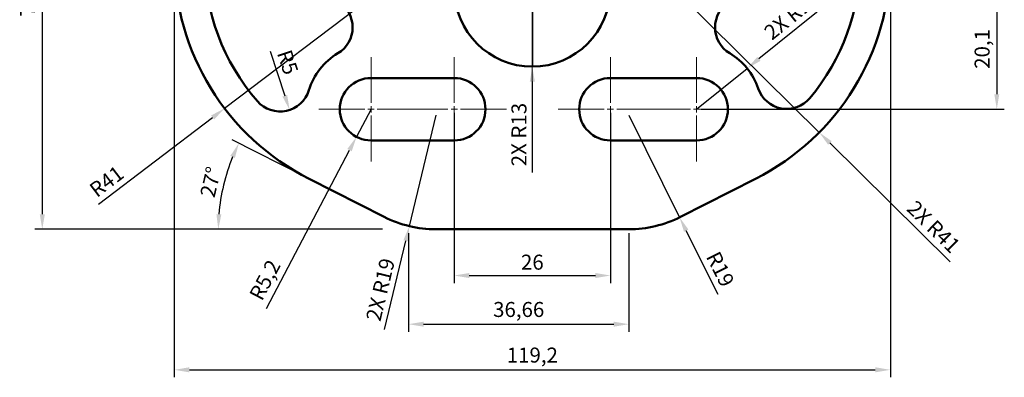
# Model space of a CAD drawing. Units: millimetres. Extents: x 11989 to 12153, y 10398 to 10572.
# Tile 1 of 2: x 11989 to 12153, y 10398 to 10458. Entities that reach past the tile are written whole.
import ezdxf

# ---------------------------------------------------------------- set-up
doc = ezdxf.new("R2010")
doc.units = ezdxf.units.MM
doc.linetypes.add('CENTER', pattern=[50.8, 31.75, -6.35, 6.35, -6.35])
for name, color, linetype, lineweight in [('M-CNTR', 1, 'CENTER', 18), ('M-CONS', 8, 'Continuous', 13), ('M-DIMS', 2, 'Continuous', 25), ('M-OUTL', 7, 'Continuous', 50)]:
    doc.layers.add(name, color=color, linetype=linetype, lineweight=lineweight)
doc.styles.get("Standard").update_dxf_attribs({"font": 'arial.ttf'})
doc.dimstyles.new('ISO-25', dxfattribs={"dimtxt": 2.5, "dimasz": 2.5, "dimexe": 1.25, "dimexo": 0.625, "dimtad": 1, "dimtxsty": 'Standard', "dimcen": 2.5, "dimadec": 0, "dimazin": 0, "dimtfac": 1, "dimtmove": 0, "dimatfit": 3, "dimfxl": 1, "dimarcsym": 0})

# ---------------------------------------------------------------- blocks, each defined once
blk = doc.blocks.new('*U1')
at = {"layer": 'M-CNTR', "color": 0, "transparency": 16777216}
for p, q in [((0, 1.04), (0, 8.7)), ((-8.7, 0), (-1.04, 0)), ((1.04, 0), (8.7, 0)), ((0, -8.7), (0, -1.04))]:
    blk.add_line(p, q, dxfattribs=at)
at = {"layer": 'M-CNTR', "color": 0, "linetype": 'Continuous', "transparency": 16777216}
for p, q in [((-0.52, 0), (0.52, 0)), ((0, -0.52), (0, 0.52))]:
    blk.add_line(p, q, dxfattribs=at)
blk = doc.blocks.new('*U2')
at = {"layer": 'M-CNTR', "color": 0, "transparency": 16777216}
for p, q in [((0, 1.04), (0, 8.7)), ((-8.7, 0), (-1.04, 0)), ((1.04, 0), (8.7, 0)), ((0, -8.7), (0, -1.04))]:
    blk.add_line(p, q, dxfattribs=at)
at = {"layer": 'M-CNTR', "color": 0, "linetype": 'Continuous', "transparency": 16777216}
for p, q in [((-0.52, 0), (0.52, 0)), ((0, -0.52), (0, 0.52))]:
    blk.add_line(p, q, dxfattribs=at)
blk = doc.blocks.new('*U3')
at = {"layer": 'M-CNTR', "color": 0, "transparency": 16777216}
for p, q in [((0, 1.04), (0, 8.7)), ((-8.7, 0), (-1.04, 0)), ((1.04, 0), (8.7, 0)), ((0, -8.7), (0, -1.04))]:
    blk.add_line(p, q, dxfattribs=at)
at = {"layer": 'M-CNTR', "color": 0, "linetype": 'Continuous', "transparency": 16777216}
for p, q in [((-0.52, 0), (0.52, 0)), ((0, -0.52), (0, 0.52))]:
    blk.add_line(p, q, dxfattribs=at)
blk = doc.blocks.new('*U4')
at = {"layer": 'M-CNTR', "color": 0, "transparency": 16777216}
for p, q in [((0, 1.04), (0, 8.7)), ((-8.7, 0), (-1.04, 0)), ((1.04, 0), (8.7, 0)), ((0, -8.7), (0, -1.04))]:
    blk.add_line(p, q, dxfattribs=at)
at = {"layer": 'M-CNTR', "color": 0, "linetype": 'Continuous', "transparency": 16777216}
for p, q in [((-0.52, 0), (0.52, 0)), ((0, -0.52), (0, 0.52))]:
    blk.add_line(p, q, dxfattribs=at)
blk = doc.blocks.new('*U12')
at = {"layer": 'M-CNTR', "color": 0, "transparency": 16777216}
for p, q in [((0, 2.6), (0, 16.5)), ((-16.5, 0), (-2.6, 0)), ((2.6, 0), (16.5, 0)), ((0, -16.5), (0, -2.6))]:
    blk.add_line(p, q, dxfattribs=at)
at = {"layer": 'M-CNTR', "color": 0, "linetype": 'Continuous', "transparency": 16777216}
for p, q in [((-1.3, 0), (1.3, 0)), ((0, -1.3), (0, 1.3))]:
    blk.add_line(p, q, dxfattribs=at)
blk = doc.blocks.new('*D13')
at = {"layer": 'Defpoints', "color": 0, "transparency": 16777216}
for p in [(12061.03, 10442.87), (12087.03, 10442.87), (12087.03, 10415.17)]:
    blk.add_point(p, dxfattribs=at)
at = {"layer": 'M-DIMS', "color": 0, "lineweight": -2, "transparency": 16777216}
for p, q in [((12061.03, 10442.25), (12061.03, 10413.92)), ((12087.03, 10442.25), (12087.03, 10413.92)), ((12063.53, 10415.17), (12084.53, 10415.17))]:
    blk.add_line(p, q, dxfattribs=at)
at = {"layer": 'M-DIMS', "color": 0, "transparency": 16777216}
for points in [[(12063.53, 10415.59), (12063.53, 10414.75), (12061.03, 10415.17)], [(12084.53, 10415.59), (12084.53, 10414.75), (12087.03, 10415.17)]]:
    blk.add_solid(points, dxfattribs=at)
at = {"layer": 'M-DIMS', "color": 0, "transparency": 16777216, "insert": (12074.03, 10417.07), "char_height": 2.5, "attachment_point": 5}
blk.add_mtext('26', dxfattribs=at)
blk = doc.blocks.new('*D14')
at = {"layer": 'Defpoints', "color": 0, "transparency": 16777216}
for p in [(12053.43, 10422.87), (12090.09, 10422.87), (12090.09, 10407.06)]:
    blk.add_point(p, dxfattribs=at)
at = {"layer": 'M-DIMS', "color": 0, "lineweight": -2, "transparency": 16777216}
for p, q in [((12053.43, 10422.25), (12053.43, 10405.81)), ((12090.09, 10422.25), (12090.09, 10405.81)), ((12055.93, 10407.06), (12087.59, 10407.06))]:
    blk.add_line(p, q, dxfattribs=at)
at = {"layer": 'M-DIMS', "color": 0, "transparency": 16777216}
for points in [[(12055.93, 10407.48), (12055.93, 10406.64), (12053.43, 10407.06)], [(12087.59, 10407.48), (12087.59, 10406.64), (12090.09, 10407.06)]]:
    blk.add_solid(points, dxfattribs=at)
at = {"layer": 'M-DIMS', "color": 0, "transparency": 16777216, "insert": (12071.76, 10409.19), "char_height": 2.5, "attachment_point": 5}
blk.add_mtext('36,66', dxfattribs=at)
blk = doc.blocks.new('*D15')
at = {"layer": 'Defpoints', "color": 0, "transparency": 16777216}
for p in [(12014.43, 10479.37), (12133.63, 10479.37), (12133.63, 10399.46)]:
    blk.add_point(p, dxfattribs=at)
at = {"layer": 'M-DIMS', "color": 0, "lineweight": -2, "transparency": 16777216}
for p, q in [((12014.43, 10478.74), (12014.43, 10398.21)), ((12133.63, 10478.74), (12133.63, 10398.21)), ((12016.93, 10399.46), (12131.13, 10399.46))]:
    blk.add_line(p, q, dxfattribs=at)
at = {"layer": 'M-DIMS', "color": 0, "transparency": 16777216}
for points in [[(12016.93, 10399.88), (12016.93, 10399.04), (12014.43, 10399.46)], [(12131.13, 10399.88), (12131.13, 10399.04), (12133.63, 10399.46)]]:
    blk.add_solid(points, dxfattribs=at)
at = {"layer": 'M-DIMS', "color": 0, "transparency": 16777216, "insert": (12074.03, 10401.59), "char_height": 2.5, "attachment_point": 5}
blk.add_mtext('119,2', dxfattribs=at)
blk = doc.blocks.new('*D27')
at = {"layer": 'Defpoints', "color": 0, "transparency": 16777216}
for p in [(12032.04, 10447.49), (12033.62, 10442.74)]:
    blk.add_point(p, dxfattribs=at)
at = {"layer": 'M-DIMS', "color": 0, "lineweight": -2, "transparency": 16777216}
blk.add_line((12030.37, 10452.52), (12032.83, 10445.12), dxfattribs=at)
at = {"layer": 'M-DIMS', "color": 0, "transparency": 16777216}
blk.add_solid([(12033.22, 10445.25), (12032.43, 10444.99), (12033.62, 10442.74)], dxfattribs=at)
at = {"layer": 'M-DIMS', "color": 0, "transparency": 16777216, "insert": (12033, 10450.6), "char_height": 2.5, "attachment_point": 5, "rotation": 288.3964}
blk.add_mtext('R5', dxfattribs=at)
blk = doc.blocks.new('*D28')
at = {"layer": 'Defpoints', "color": 0, "transparency": 16777216}
for p in [(12047.18, 10442.87), (12044.76, 10438.27)]:
    blk.add_point(p, dxfattribs=at)
at = {"layer": 'M-DIMS', "color": 0, "lineweight": -2, "transparency": 16777216}
for p, q in [((12047.18, 10442.87), (12044.76, 10438.27)), ((12029.77, 10409.68), (12043.6, 10436.05))]:
    blk.add_line(p, q, dxfattribs=at)
at = {"layer": 'M-DIMS', "color": 0, "transparency": 16777216}
blk.add_solid([(12043.23, 10436.25), (12043.97, 10435.86), (12044.76, 10438.27)], dxfattribs=at)
at = {"layer": 'M-DIMS', "color": 0, "transparency": 16777216, "insert": (12029.79, 10414.28), "char_height": 2.5, "attachment_point": 5, "rotation": 62.3298}
blk.add_mtext('R5,2', dxfattribs=at)
blk = doc.blocks.new('*D29')
at = {"layer": 'Defpoints', "color": 0, "transparency": 16777216}
for p in [(12023.29, 10432.63), (12036.88, 10431.27), (12049.38, 10424.93), (12049.73, 10422.87), (12053.43, 10422.87)]:
    blk.add_point(p, dxfattribs=at)
at = {"layer": 'M-DIMS', "color": 0, "lineweight": -2, "transparency": 16777216}
for p, q in [((12036.32, 10431.55), (12024.06, 10437.77)), ((12049.11, 10422.87), (12020.5, 10422.87))]:
    blk.add_line(p, q, dxfattribs=at)
blk.add_arc((12053.43, 10422.87), 31.68, 157.6226, 175.4774, dxfattribs=at)
at = {"layer": 'M-DIMS', "color": 0, "transparency": 16777216}
for points in [[(12023.76, 10435.11), (12024.51, 10434.76), (12025.18, 10437.21)], [(12022.26, 10425.35), (12021.43, 10425.39), (12021.75, 10422.87)]]:
    blk.add_solid(points, dxfattribs=at)
at = {"layer": 'M-DIMS', "color": 0, "transparency": 16777216, "insert": (12020.79, 10430.68), "char_height": 2.5, "attachment_point": 5, "rotation": 76.55}
blk.add_mtext('27°', dxfattribs=at)
blk = doc.blocks.new('*D30')
at = {"layer": 'Defpoints', "color": 0, "transparency": 16777216}
for p in [(12055.43, 10467.83), (12022.79, 10443.01)]:
    blk.add_point(p, dxfattribs=at)
at = {"layer": 'M-DIMS', "color": 0, "lineweight": -2, "transparency": 16777216}
for p, q in [((12055.43, 10467.83), (12022.79, 10443.01)), ((12001.8, 10427.05), (12020.8, 10441.5))]:
    blk.add_line(p, q, dxfattribs=at)
at = {"layer": 'M-DIMS', "color": 0, "transparency": 16777216}
blk.add_solid([(12020.55, 10441.83), (12021.06, 10441.17), (12022.79, 10443.01)], dxfattribs=at)
at = {"layer": 'M-DIMS', "color": 0, "transparency": 16777216, "insert": (12003.35, 10430.59), "char_height": 2.5, "attachment_point": 5, "rotation": 37.2506}
blk.add_mtext('R41', dxfattribs=at)
blk = doc.blocks.new('*D31')
at = {"layer": 'Defpoints', "color": 0, "transparency": 16777216}
for p in [(12090.09, 10441.87), (12098.54, 10424.86)]:
    blk.add_point(p, dxfattribs=at)
at = {"layer": 'M-DIMS', "color": 0, "lineweight": -2, "transparency": 16777216}
for p, q in [((12090.09, 10441.87), (12098.54, 10424.86)), ((12104.94, 10411.99), (12099.66, 10422.62))]:
    blk.add_line(p, q, dxfattribs=at)
at = {"layer": 'M-DIMS', "color": 0, "transparency": 16777216}
blk.add_solid([(12100.03, 10422.81), (12099.28, 10422.44), (12098.54, 10424.86)], dxfattribs=at)
at = {"layer": 'M-DIMS', "color": 0, "transparency": 16777216, "insert": (12105.04, 10416.08), "char_height": 2.5, "attachment_point": 5, "rotation": 296.4371}
blk.add_mtext('R19', dxfattribs=at)
blk = doc.blocks.new('*D33')
at = {"layer": 'Defpoints', "color": 0, "transparency": 16777216}
for p in [(11992.68, 10500.37), (11992.45, 10422.87), (12049.1, 10422.87)]:
    blk.add_point(p, dxfattribs=at)
at = {"layer": 'M-DIMS', "color": 0, "lineweight": -2, "transparency": 16777216}
for p, q in [((11992.06, 10500.37), (11991.2, 10500.37)), ((11992.45, 10497.87), (11992.45, 10425.37)), ((12048.47, 10422.87), (11991.2, 10422.87))]:
    blk.add_line(p, q, dxfattribs=at)
at = {"layer": 'M-DIMS', "color": 0, "transparency": 16777216}
for points in [[(11992.03, 10497.87), (11992.87, 10497.87), (11992.45, 10500.37)], [(11992.03, 10425.37), (11992.87, 10425.37), (11992.45, 10422.87)]]:
    blk.add_solid(points, dxfattribs=at)
at = {"layer": 'M-DIMS', "color": 0, "transparency": 16777216, "insert": (11990.33, 10461.62), "char_height": 2.5, "attachment_point": 5, "rotation": 90}
blk.add_mtext('77,5', dxfattribs=at)
blk = doc.blocks.new('*D37')
at = {"layer": 'Defpoints', "color": 0, "transparency": 16777216}
for p in [(12102.04, 10462.97), (12101.38, 10442.87), (12151.35, 10442.87)]:
    blk.add_point(p, dxfattribs=at)
at = {"layer": 'M-DIMS', "color": 0, "lineweight": -2, "transparency": 16777216}
for p, q in [((12102.66, 10462.97), (12152.6, 10462.97)), ((12151.35, 10460.47), (12151.35, 10445.37)), ((12102, 10442.87), (12152.6, 10442.87))]:
    blk.add_line(p, q, dxfattribs=at)
at = {"layer": 'M-DIMS', "color": 0, "transparency": 16777216}
for points in [[(12150.94, 10460.47), (12151.77, 10460.47), (12151.35, 10462.97)], [(12150.94, 10445.37), (12151.77, 10445.37), (12151.35, 10442.87)]]:
    blk.add_solid(points, dxfattribs=at)
at = {"layer": 'M-DIMS', "color": 0, "transparency": 16777216, "insert": (12149.23, 10452.92), "char_height": 2.5, "attachment_point": 5, "rotation": 90}
blk.add_mtext('20,1', dxfattribs=at)
blk = doc.blocks.new('*D40')
at = {"layer": 'Defpoints', "color": 0, "transparency": 16777216}
for p in [(12092.63, 10467.83), (12121.79, 10439.01)]:
    blk.add_point(p, dxfattribs=at)
at = {"layer": 'M-DIMS', "color": 0, "lineweight": -2, "transparency": 16777216}
for p, q in [((12092.63, 10467.83), (12121.79, 10439.01)), ((12143.61, 10417.44), (12123.57, 10437.25))]:
    blk.add_line(p, q, dxfattribs=at)
at = {"layer": 'M-DIMS', "color": 0, "transparency": 16777216}
blk.add_solid([(12123.86, 10437.55), (12123.27, 10436.96), (12121.79, 10439.01)], dxfattribs=at)
at = {"layer": 'M-DIMS', "color": 0, "transparency": 16777216, "insert": (12140.61, 10423.06), "char_height": 2.5, "attachment_point": 5, "rotation": 315.3343}
blk.add_mtext('2X R41', dxfattribs=at)
blk = doc.blocks.new('*D43')
at = {"layer": 'Defpoints', "color": 0, "transparency": 16777216}
for p in [(12109.8, 10449.68), (12101.38, 10442.87)]:
    blk.add_point(p, dxfattribs=at)
at = {"layer": 'M-DIMS', "color": 0, "lineweight": -2, "transparency": 16777216}
for p, q in [((12127.29, 10463.82), (12111.74, 10451.25)), ((12101.38, 10442.87), (12109.8, 10449.68))]:
    blk.add_line(p, q, dxfattribs=at)
at = {"layer": 'M-DIMS', "color": 0, "transparency": 16777216}
blk.add_solid([(12111.48, 10451.58), (12112.01, 10450.93), (12109.8, 10449.68)], dxfattribs=at)
at = {"layer": 'M-DIMS', "color": 0, "transparency": 16777216, "insert": (12119.29, 10459.8), "char_height": 2.5, "attachment_point": 5, "rotation": 38.9595}
blk.add_mtext('2X R10.83', dxfattribs=at)
blk = doc.blocks.new('*D47')
at = {"layer": 'Defpoints', "color": 0, "transparency": 16777216}
for p in [(12074.03, 10462.97), (12074.03, 10449.97)]:
    blk.add_point(p, dxfattribs=at)
at = {"layer": 'M-DIMS', "color": 0, "lineweight": -2, "transparency": 16777216}
for p, q in [((12074.03, 10462.97), (12074.03, 10449.97)), ((12074.03, 10432.33), (12074.03, 10447.47))]:
    blk.add_line(p, q, dxfattribs=at)
at = {"layer": 'M-DIMS', "color": 0, "transparency": 16777216}
blk.add_solid([(12073.61, 10447.47), (12074.45, 10447.47), (12074.03, 10449.97)], dxfattribs=at)
at = {"layer": 'M-DIMS', "color": 0, "transparency": 16777216, "insert": (12072.13, 10438.65), "char_height": 2.5, "attachment_point": 5, "rotation": 89.998}
blk.add_mtext('2X R13', dxfattribs=at)
blk = doc.blocks.new('*D49')
at = {"layer": 'Defpoints', "color": 0, "transparency": 16777216}
for p in [(12057.97, 10441.87), (12053.55, 10423.39)]:
    blk.add_point(p, dxfattribs=at)
at = {"layer": 'M-DIMS', "color": 0, "lineweight": -2, "transparency": 16777216}
for p, q in [((12057.97, 10441.87), (12053.55, 10423.39)), ((12049.43, 10406.16), (12052.97, 10420.96))]:
    blk.add_line(p, q, dxfattribs=at)
at = {"layer": 'M-DIMS', "color": 0, "transparency": 16777216}
blk.add_solid([(12052.57, 10421.06), (12053.38, 10420.86), (12053.55, 10423.39)], dxfattribs=at)
at = {"layer": 'M-DIMS', "color": 0, "transparency": 16777216, "insert": (12049.05, 10412.75), "char_height": 2.5, "attachment_point": 5, "rotation": 76.55}
blk.add_mtext('2X R19', dxfattribs=at)

msp = doc.modelspace()

# ---------------------------------------------------------------- linework, layer by layer
at = {"layer": 'M-CONS'}
for q in [(12057.9734, 10422.8722), (12090.0855, 10422.8722)]:
    msp.add_line((12074.0295, 10422.8722), q, dxfattribs=at)
at = {"layer": 'M-OUTL'}
for p, q in [((12047.1795, 10448.0722), (12061.0295, 10448.0722)), ((12087.0295, 10448.0722), (12101.3795, 10448.0722)), ((12047.1795, 10437.6722), (12061.0295, 10437.6722)), ((12087.0295, 10437.6722), (12101.3795, 10437.6722)), ((12049.3772, 10424.9281), (12036.8796, 10431.2684)), ((12098.6817, 10424.9281), (12111.1793, 10431.2684)), ((12090.0855, 10422.8722), (12057.9734, 10422.8722))]:
    msp.add_line(p, q, dxfattribs=at)
for points in [[(12046.708, 10545.9953), (12018.9938, 10505.6215, 0.15153611), (12014.4295, 10490.9071), (12014.4295, 10467.8321, 0.28250026), (12036.8796, 10431.2684)], [(12101.3509, 10545.9953), (12129.0651, 10505.6215, -0.15153611), (12133.6295, 10490.9071), (12133.6295, 10467.8321, -0.28250026), (12111.1793, 10431.2684)], [(12046.145, 10536.3402), (12023.116, 10502.7918, 0.15153611), (12019.4295, 10490.9071), (12019.4295, 10467.8321, 0.18088402), (12028.2649, 10444.2082, 0.18088402)], [(12101.9139, 10536.3402), (12124.9429, 10502.7918, -0.15153611), (12128.6295, 10490.9071), (12128.6295, 10467.8321, -0.17622487), (12120.2162, 10444.7027, -0.17622487)]]:
    msp.add_lwpolyline(points, format="xyb", dxfattribs=at)
for centre, radius, start, end in [((12074.0295, 10462.9722), 13, 180, 0), ((12039.1076, 10456.4896), 5, 300.657568, 59.277925), ((12109.4513, 10456.4896), 5, 120.722075, 239.342432), ((12047.1795, 10442.8722), 10.83, 120.657568, 163.042064), ((12101.3795, 10442.8722), 10.83, 18.576209, 59.342432), ((12047.1795, 10442.8722), 5.2, 90, 270), ((12061.0295, 10442.8722), 5.2, 270, 90), ((12087.0295, 10442.8722), 5.2, 90, 270), ((12101.3795, 10442.8722), 5.2, 270, 90), ((12032.0378, 10447.4893), 5, 221.012109, 343.042064), ((12116.3847, 10447.9151), 5, 198.576209, 320.022696), ((12057.9734, 10441.8722), 19, 243.1, 270), ((12090.0855, 10441.8722), 19, 270, 296.9)]:
    msp.add_arc(centre, radius, start, end, dxfattribs=at)

# ---------------------------------------------------------------- block references
at = {"layer": 'M-CNTR'}
for name, p in [('*U12', (12074.0295, 10462.9722)), ('*U4', (12047.1795, 10442.8722)), ('*U1', (12061.0295, 10442.8722)), ('*U2', (12087.0295, 10442.8722)), ('*U3', (12101.3795, 10442.8722))]:
    msp.add_blockref(name, p, dxfattribs=at)

# ---------------------------------------------------------------- dimensions: what is measured, and where the dimension line sits
at = {"layer": 'M-DIMS'}
for base, p1, p2, picture, middle in [((11992.4491, 10422.8722), (11992.6842, 10500.3722), (12049.0984, 10422.8722), '*D33', (11990.3268, 10461.6222)), ((12151.353, 10442.8722), (12102.036, 10462.9735), (12101.3795, 10442.8722), '*D37', (12149.2256, 10452.9229))]:
    dim = msp.add_linear_dim(base=base, p1=p1, p2=p2, angle=90, dimstyle='ISO-25', override={"dimclrd": 0, "dimclre": 0, "dimclrt": 0}, dxfattribs=at)
    dim.commit()
    dim.dimension.update_dxf_attribs({"geometry": picture, "text_midpoint": middle})
for base, p1, p2, picture, middle in [((12133.6295, 10399.4601), (12014.4295, 10479.3696), (12133.6295, 10479.3696), '*D15', (12074.0295, 10401.5875)), ((12087.0295, 10415.1708), (12061.0295, 10442.8722), (12087.0295, 10442.8722), '*D13', (12074.0295, 10417.0722)), ((12090.0855, 10407.0584), (12053.4295, 10422.8722), (12090.0855, 10422.8722), '*D14', (12071.7575, 10409.1858))]:
    dim = msp.add_linear_dim(base=base, p1=p1, p2=p2, dimstyle='ISO-25', override={"dimclrd": 0, "dimclre": 0, "dimclrt": 0}, dxfattribs=at)
    dim.commit()
    dim.dimension.update_dxf_attribs({"geometry": picture, "text_midpoint": middle})
for center, mpoint, picture, middle in [((12055.4295, 10467.8321), (12022.7936, 10443.0147), '*D30', (12004.4846, 10429.0919)), ((12032.0378, 10447.4893), (12033.6157, 10442.7449), '*D27', (12031.2014, 10450.004)), ((12047.1795, 10442.8722), (12044.7647, 10438.2669), '*D28', (12031.6702, 10413.2941)), ((12090.0855, 10441.8722), (12098.5446, 10424.8592), '*D31', (12103.3327, 10415.2293))]:
    dim = msp.add_radius_dim(center=center, mpoint=mpoint, dimstyle='ISO-25', override={"dimclrd": 0, "dimclre": 0, "dimclrt": 0}, dxfattribs=at)
    dim.commit()
    dim.dimension.update_dxf_attribs({"geometry": picture, "text_midpoint": middle, "dimtype": 164})
for center, mpoint, picture, middle in [((12092.6295, 10467.8321), (12121.7895, 10439.0104), '*D40', (12139.2855, 10421.7173)), ((12057.9734, 10441.8722), (12053.5541, 10423.3933), '*D49', (12050.9025, 10412.306))]:
    dim = msp.add_radius_dim(center=center, mpoint=mpoint, text='2X <>', dimstyle='ISO-25', override={"dimdec": 0, "dimlfac": 1, "dimrnd": 0, "dimzin": 0, "dimdsep": 46, "dimlunit": 2}, dxfattribs=at)
    dim.commit()
    dim.dimension.update_dxf_attribs({"geometry": picture, "text_midpoint": middle, "dimtype": 164})
for center, mpoint, override, picture, middle in [((12101.3795, 10442.8722), (12109.8008, 10449.6818), {"dimdec": 2, "dimlfac": 1, "dimrnd": 0, "dimzin": 0, "dimdsep": 46, "dimlunit": 2}, '*D43', (12119.2939, 10459.8045)), ((12074.0295, 10462.9722), (12074.029, 10449.9722), {"dimdec": 0, "dimlfac": 1, "dimrnd": 0, "dimzin": 0, "dimdsep": 46, "dimlunit": 2}, '*D47', (12072.1263, 10438.6532))]:
    dim = msp.add_radius_dim(center=center, mpoint=mpoint, text='2X <>', dimstyle='ISO-25', override=override, dxfattribs=at)
    dim.commit()
    dim.dimension.update_dxf_attribs({"geometry": picture, "text_midpoint": middle})
dim = msp.add_angular_dim_2l(base=(12023.2885, 10432.6268), line1=((12053.4295, 10422.8722), (12049.7327, 10422.8722)), line2=((12049.3772, 10424.9281), (12036.8796, 10431.2684)), dimstyle='ISO-25', override={"dimclrd": 0, "dimclre": 0, "dimclrt": 0}, dxfattribs=at)
dim.commit()
dim.dimension.update_dxf_attribs({"geometry": '*D29', "text_midpoint": (12020.7897, 10430.6782)})

doc.saveas('drawing.dxf')
